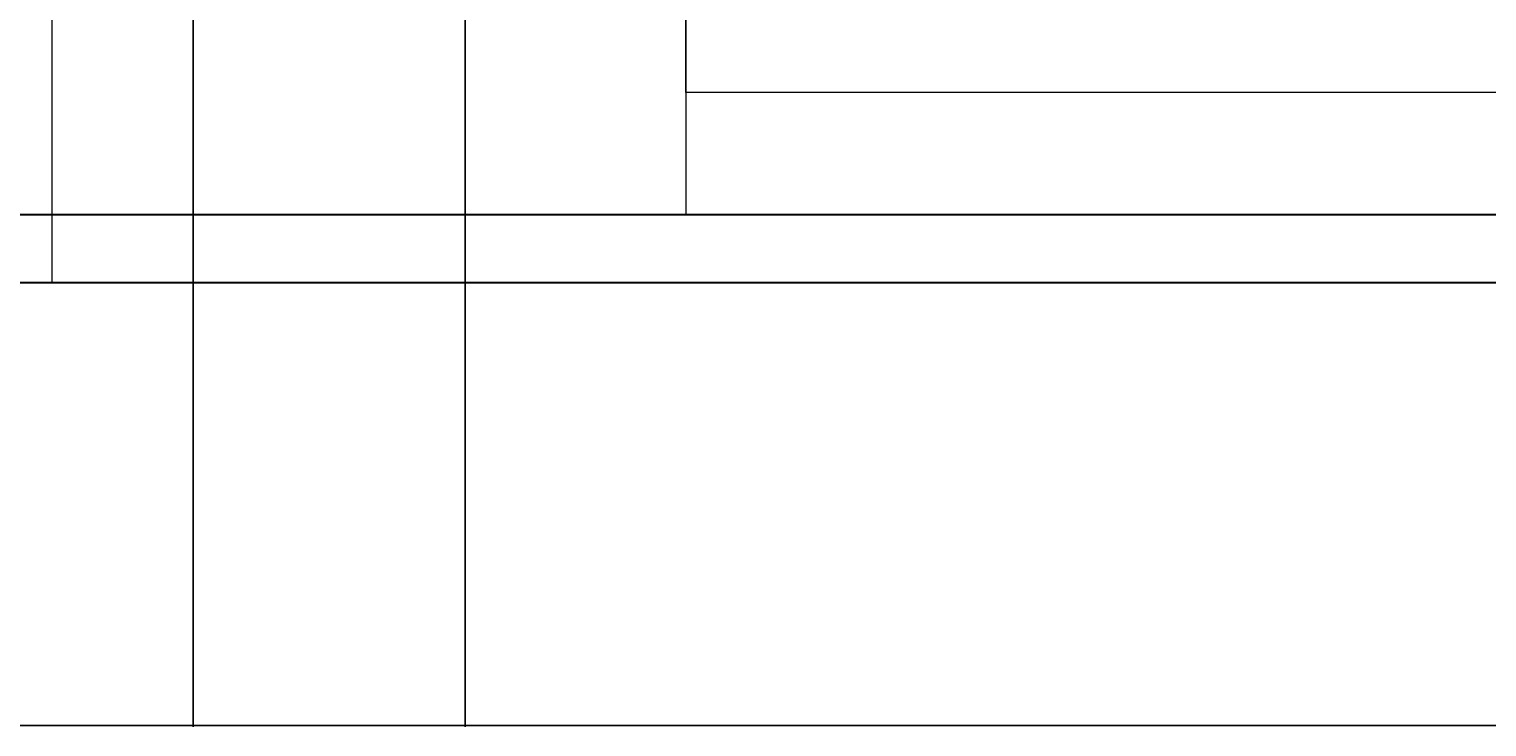
# Model space of a CAD drawing. Units: inches. Extents: x -46 to 1145, y -527 to 760.
# Tile 2 of 57: x 187 to 380, y -527 to -435. Entities that reach past the tile are written whole.
import ezdxf

# ---------------------------------------------------------------- set-up
doc = ezdxf.new("R2010")
doc.units = ezdxf.units.IN
doc.header["$MEASUREMENT"] = 0
for name, color, linetype, lineweight in [('A-ANNO-DIMS', 2, 'Continuous', 18), ('C-PKNG', 8, 'Continuous', 18), ('C-ROAD', 9, 'Continuous', 18), ('C-SITE', 7, 'Continuous', 30)]:
    doc.layers.add(name, color=color, linetype=linetype, lineweight=lineweight)
doc.styles.get("Standard").update_dxf_attribs({"font": 'arial.ttf'})
doc.dimstyles.get("Standard").update_dxf_attribs({"dimtxt": 0.18, "dimasz": 0.18, "dimexe": 0.18, "dimexo": 0.0625, "dimgap": 0.09, "dimtad": 0, "dimtih": 1, "dimtoh": 1, "dimdec": 0, "dimzin": 0, "dimdsep": 46, "dimlunit": 3, "dimtxsty": 'Standard', "dimcen": 0.09, "dimadec": 0, "dimazin": 0, "dimtfac": 1, "dimtdec": 0, "dimtofl": 0, "dimtmove": 0, "dimatfit": 3, "dimfxl": 1, "dimtolj": 1, "dimtzin": 0, "dimarcsym": 0})

# ---------------------------------------------------------------- blocks, each defined once
blk = doc.blocks.new('*D684')
at = {"layer": 'A-ANNO-DIMS', "color": 0, "lineweight": -2, "transparency": 16777216}
for p, q in [((12.56, -468.54), (12.56, -527.26)), ((1086.56, -468.54), (1086.56, -527.26)), ((12.74, -527.08), (549.21, -527.08)), ((1086.38, -527.08), (549.91, -527.08))]:
    blk.add_line(p, q, dxfattribs=at)
at = {"layer": 'A-ANNO-DIMS', "color": 0, "transparency": 16777216}
for points in [[(12.74, -527.05), (12.74, -527.11), (12.56, -527.08)], [(1086.38, -527.05), (1086.38, -527.11), (1086.56, -527.08)]]:
    blk.add_solid(points, dxfattribs=at)
at = {"layer": 'Defpoints', "color": 0, "transparency": 16777216}
for p in [(12.56, -468.48), (1086.56, -468.48), (1086.56, -527.08)]:
    blk.add_point(p, dxfattribs=at)
at = {"layer": 'A-ANNO-DIMS', "color": 0, "transparency": 16777216, "insert": (549.56, -527.08), "char_height": 0.18, "attachment_point": 5}
blk.add_mtext('\\A1;1074', dxfattribs=at)
blk = doc.blocks.new('*D695')
at = {"layer": 'A-ANNO-DIMS', "color": 0, "lineweight": -2, "transparency": 16777216}
for p, q in [((208.27, 221.46), (208.27, -527.26)), ((244.27, 221.46), (244.27, -527.26)), ((208.45, -527.08), (226.05, -527.08)), ((244.09, -527.08), (226.49, -527.08))]:
    blk.add_line(p, q, dxfattribs=at)
at = {"layer": 'A-ANNO-DIMS', "color": 0, "transparency": 16777216}
for points in [[(208.45, -527.05), (208.45, -527.11), (208.27, -527.08)], [(244.09, -527.05), (244.09, -527.11), (244.27, -527.08)]]:
    blk.add_solid(points, dxfattribs=at)
at = {"layer": 'Defpoints', "color": 0, "transparency": 16777216}
for p in [(208.27, 221.52), (244.27, 221.52), (244.27, -527.08)]:
    blk.add_point(p, dxfattribs=at)
at = {"layer": 'A-ANNO-DIMS', "color": 0, "transparency": 16777216, "insert": (226.27, -527.08), "char_height": 0.18, "attachment_point": 5}
blk.add_mtext('\\A1;36', dxfattribs=at)
blk = doc.blocks.new('*D702')
at = {"layer": 'A-ANNO-DIMS', "color": 0, "lineweight": -2, "transparency": 16777216}
for p, q in [((189.63, -39.48), (1145.34, -39.48)), ((1145.16, -39.66), (1145.16, -249.3)), ((1145.16, -459.3), (1145.16, -249.66)), ((183.63, -459.48), (1145.34, -459.48))]:
    blk.add_line(p, q, dxfattribs=at)
at = {"layer": 'A-ANNO-DIMS', "color": 0, "transparency": 16777216}
for points in [[(1145.13, -39.66), (1145.19, -39.66), (1145.16, -39.48)], [(1145.13, -459.3), (1145.19, -459.3), (1145.16, -459.48)]]:
    blk.add_solid(points, dxfattribs=at)
at = {"layer": 'Defpoints', "color": 0, "transparency": 16777216}
for p in [(189.56, -39.48), (1145.16, -39.48), (183.56, -459.48)]:
    blk.add_point(p, dxfattribs=at)
at = {"layer": 'A-ANNO-DIMS', "color": 0, "transparency": 16777216, "insert": (1145.16, -249.48), "char_height": 0.18, "attachment_point": 5}
blk.add_mtext('\\A1;420', dxfattribs=at)

msp = doc.modelspace()

# ---------------------------------------------------------------- linework, layer by layer
at = {"layer": 'C-PKNG'}
msp.add_line((273.5156, -39.4824), (273.5156, -459.4824), dxfattribs=at)
msp.add_lwpolyline([(501.7297, -443.2988), (273.5156, -443.2988), (273.5156, -345.0009), (501.7297, -345.0009)], close=True, dxfattribs=at)
at = {"layer": 'C-ROAD'}
msp.add_line((189.5637, 221.5176), (189.5637, -468.4824), dxfattribs=at)
at = {"layer": 'C-SITE'}
for p, q in [((21.5637, -459.4824), (1077.5637, -459.4824)), ((12.5637, -468.4824), (1086.5637, -468.4824))]:
    msp.add_line(p, q, dxfattribs=at)

# ---------------------------------------------------------------- dimensions: what is measured, and where the dimension line sits
at = {"layer": 'A-ANNO-DIMS'}
for base, p1, p2, picture, middle in [((244.2731, -527.0824), (208.2731, 221.5176), (244.2731, 221.5176), '*D695', (226.2731, -527.0824)), ((1086.5637, -527.0824), (12.5637, -468.4824), (1086.5637, -468.4824), '*D684', (549.5637, -527.0824))]:
    dim = msp.add_linear_dim(base=base, p1=p1, p2=p2, dimstyle='Standard', override={"dimdec": 0, "dimlfac": 1, "dimrnd": 0, "dimzin": 0, "dimdsep": 46, "dimlunit": 2}, dxfattribs=at)
    dim.commit()
    dim.dimension.update_dxf_attribs({"geometry": picture, "text_midpoint": middle})
dim = msp.add_linear_dim(base=(1145.1637, -39.4824), p1=(183.5637, -459.4824), p2=(189.5637, -39.4824), angle=90, dimstyle='Standard', override={"dimdec": 0, "dimlfac": 1, "dimrnd": 0, "dimzin": 0, "dimdsep": 46, "dimlunit": 2}, dxfattribs=at)
dim.commit()
dim.dimension.update_dxf_attribs({"geometry": '*D702', "text_midpoint": (1145.1637, -249.4824)})

doc.saveas('drawing.dxf')
